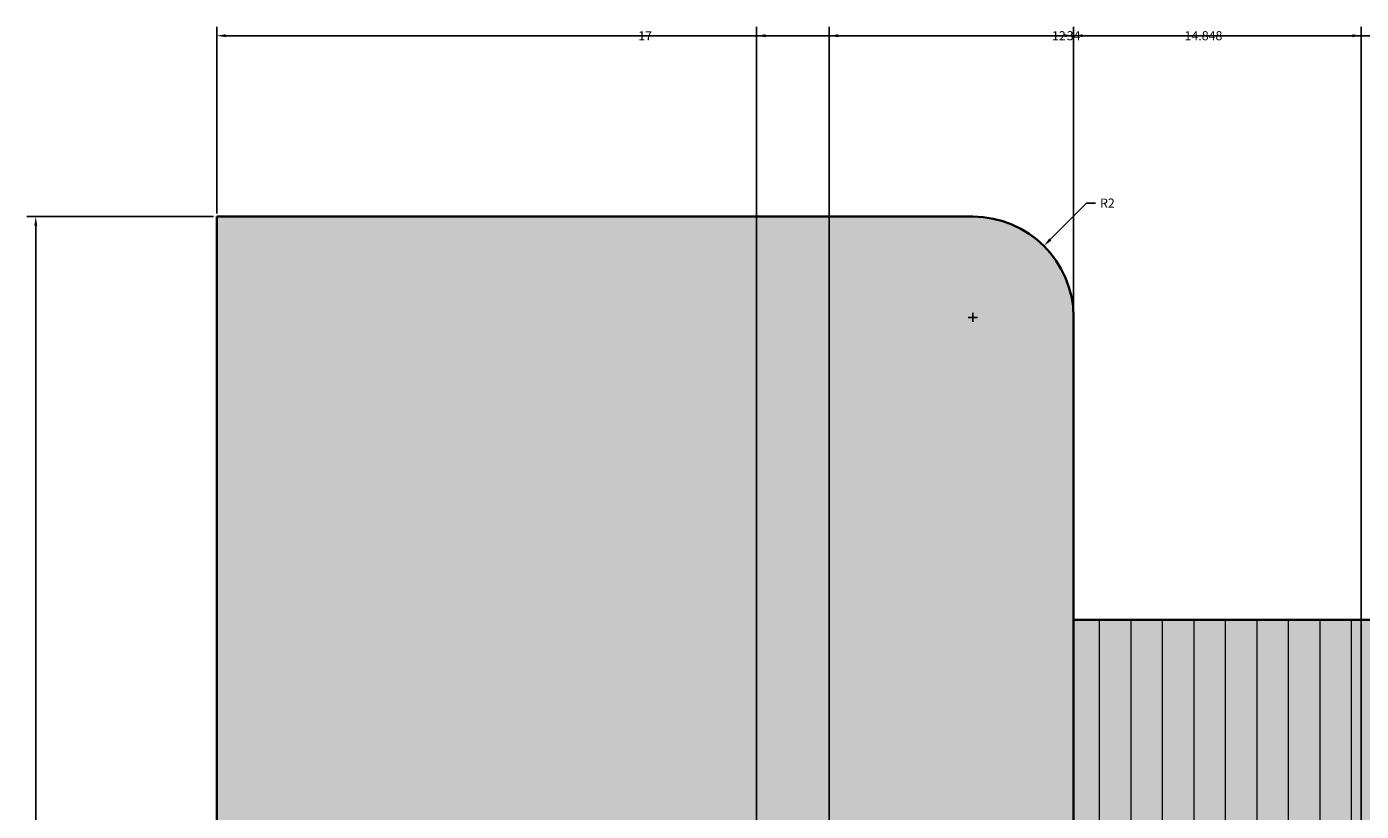
# Model space of a CAD drawing. Units: inches. Extents: x 18 to 59.8, y 2.7 to 81.2.
# Tile 8 of 9: x 18.1 to 44.6, y 65.6 to 81.2. Entities that reach past the tile are written whole.
import ezdxf

# ---------------------------------------------------------------- set-up
doc = ezdxf.new("R2010")
doc.units = ezdxf.units.IN
doc.header["$MEASUREMENT"] = 0
for name, color, linetype, lineweight in [('A-ANNO-DIMS', 2, 'Continuous', 18), ('A-ELEV', 7, 'Continuous', 35), ('A-ELEV-PATT', 8, 'Continuous', 13)]:
    doc.layers.add(name, color=color, linetype=linetype, lineweight=lineweight)
doc.styles.get("Standard").update_dxf_attribs({"font": 'arial.ttf'})
doc.dimstyles.get("Standard").update_dxf_attribs({"dimtxt": 0.18, "dimasz": 0.18, "dimexe": 0.18, "dimexo": 0.0625, "dimgap": 0.09, "dimtad": 0, "dimtih": 1, "dimtoh": 1, "dimdec": 1, "dimzin": 0, "dimdsep": 46, "dimlunit": 3, "dimtxsty": 'Standard', "dimcen": 0.09, "dimadec": 0, "dimazin": 0, "dimtfac": 1, "dimtdec": 1, "dimtofl": 0, "dimtmove": 0, "dimatfit": 3, "dimfxl": 1, "dimtolj": 1, "dimtzin": 0, "dimarcsym": 0})

# ---------------------------------------------------------------- blocks, each defined once
blk = doc.blocks.new('*D10')
at = {"layer": 'A-ANNO-DIMS', "color": 0, "lineweight": -2, "transparency": 16777216}
for p, q in [((21.86, 77.503), (21.86, 81.211)), ((22.04, 81.031), (38.641, 81.031)), ((55.68, 81.031), (39.078, 81.031)), ((55.86, 77.503), (55.86, 81.211))]:
    blk.add_line(p, q, dxfattribs=at)
at = {"layer": 'A-ANNO-DIMS', "color": 0, "transparency": 16777216}
for points in [[(22.04, 81.061), (22.04, 81.001), (21.86, 81.031)], [(55.68, 81.061), (55.68, 81.001), (55.86, 81.031)]]:
    blk.add_solid(points, dxfattribs=at)
at = {"layer": 'Defpoints', "color": 0, "transparency": 16777216}
for p in [(55.86, 81.031), (21.86, 77.441), (55.86, 77.441)]:
    blk.add_point(p, dxfattribs=at)
at = {"layer": 'A-ANNO-DIMS', "color": 0, "transparency": 16777216, "insert": (38.86, 81.031), "char_height": 0.18, "attachment_point": 5}
blk.add_mtext('\\A1;34', dxfattribs=at)
blk = doc.blocks.new('*D11')
at = {"layer": 'A-ANNO-DIMS', "color": 0, "lineweight": -2, "transparency": 16777216}
for p, q in [((21.86, 77.503), (21.86, 81.211)), ((22.04, 81.031), (30.15, 81.031)), ((38.68, 81.031), (30.57, 81.031)), ((38.86, 75.515), (38.86, 81.211))]:
    blk.add_line(p, q, dxfattribs=at)
at = {"layer": 'A-ANNO-DIMS', "color": 0, "transparency": 16777216}
for points in [[(22.04, 81.061), (22.04, 81.001), (21.86, 81.031)], [(38.68, 81.061), (38.68, 81.001), (38.86, 81.031)]]:
    blk.add_solid(points, dxfattribs=at)
at = {"layer": 'Defpoints', "color": 0, "transparency": 16777216}
for p in [(38.86, 81.031), (21.86, 77.441), (38.86, 75.452)]:
    blk.add_point(p, dxfattribs=at)
at = {"layer": 'A-ANNO-DIMS', "color": 0, "transparency": 16777216, "insert": (30.36, 81.031), "char_height": 0.18, "attachment_point": 5}
blk.add_mtext('\\A1;17', dxfattribs=at)
blk = doc.blocks.new('*D12')
at = {"layer": 'A-ANNO-DIMS', "color": 0, "lineweight": -2, "transparency": 16777216}
for p, q in [((38.86, 69.503), (38.86, 81.211)), ((39.04, 81.031), (45.765, 81.031)), ((53.26, 81.031), (46.535, 81.031)), ((53.44, 69.503), (53.44, 81.211))]:
    blk.add_line(p, q, dxfattribs=at)
at = {"layer": 'A-ANNO-DIMS', "color": 0, "transparency": 16777216}
for points in [[(39.04, 81.061), (39.04, 81.001), (38.86, 81.031)], [(53.26, 81.061), (53.26, 81.001), (53.44, 81.031)]]:
    blk.add_solid(points, dxfattribs=at)
at = {"layer": 'Defpoints', "color": 0, "transparency": 16777216}
for p in [(53.44, 81.031), (38.86, 69.441), (53.44, 69.441)]:
    blk.add_point(p, dxfattribs=at)
at = {"layer": 'A-ANNO-DIMS', "color": 0, "transparency": 16777216, "insert": (46.15, 81.031), "char_height": 0.18, "attachment_point": 5}
blk.add_mtext('\\A1;14.58', dxfattribs=at)
blk = doc.blocks.new('*D14')
at = {"layer": 'A-ANNO-DIMS', "color": 0, "lineweight": -2, "transparency": 16777216}
for p, q in [((21.797, 77.441), (18.09, 77.441)), ((18.27, 77.261), (18.27, 42.121)), ((18.27, 6.621), (18.27, 41.76)), ((21.797, 6.441), (18.09, 6.441))]:
    blk.add_line(p, q, dxfattribs=at)
at = {"layer": 'A-ANNO-DIMS', "color": 0, "transparency": 16777216}
for points in [[(18.24, 77.261), (18.3, 77.261), (18.27, 77.441)], [(18.24, 6.621), (18.3, 6.621), (18.27, 6.441)]]:
    blk.add_solid(points, dxfattribs=at)
at = {"layer": 'Defpoints', "color": 0, "transparency": 16777216}
for p in [(18.27, 77.441), (21.86, 77.441), (21.86, 6.441)]:
    blk.add_point(p, dxfattribs=at)
at = {"layer": 'A-ANNO-DIMS', "color": 0, "transparency": 16777216, "insert": (18.27, 41.941), "char_height": 0.18, "attachment_point": 5}
blk.add_mtext('\\A1;71', dxfattribs=at)
blk = doc.blocks.new('*D51')
at = {"layer": 'A-ANNO-DIMS', "color": 0, "lineweight": -2, "transparency": 16777216}
for p, q in [((34.012, 44.503), (34.012, 81.211)), ((34.192, 81.031), (40.98, 81.031)), ((48.68, 81.031), (41.891, 81.031)), ((48.86, 43.503), (48.86, 81.211))]:
    blk.add_line(p, q, dxfattribs=at)
at = {"layer": 'A-ANNO-DIMS', "color": 0, "transparency": 16777216}
for points in [[(34.192, 81.061), (34.192, 81.001), (34.012, 81.031)], [(48.68, 81.061), (48.68, 81.001), (48.86, 81.031)]]:
    blk.add_solid(points, dxfattribs=at)
at = {"layer": 'Defpoints', "color": 0, "transparency": 16777216}
for p in [(48.86, 81.031), (34.012, 44.441), (48.86, 43.441)]:
    blk.add_point(p, dxfattribs=at)
at = {"layer": 'A-ANNO-DIMS', "color": 0, "transparency": 16777216, "insert": (41.436, 81.031), "char_height": 0.18, "attachment_point": 5}
blk.add_mtext('\\A1;14.848', dxfattribs=at)
blk = doc.blocks.new('*D62')
at = {"layer": 'A-ANNO-DIMS', "color": 0, "lineweight": -2, "transparency": 16777216}
for p, q in [((32.567, 57.203), (32.567, 81.211)), ((32.747, 81.031), (38.358, 81.031)), ((44.387, 81.031), (38.777, 81.031)), ((44.567, 57.203), (44.567, 81.211))]:
    blk.add_line(p, q, dxfattribs=at)
at = {"layer": 'A-ANNO-DIMS', "color": 0, "transparency": 16777216}
for points in [[(32.747, 81.061), (32.747, 81.001), (32.567, 81.031)], [(44.387, 81.061), (44.387, 81.001), (44.567, 81.031)]]:
    blk.add_solid(points, dxfattribs=at)
at = {"layer": 'Defpoints', "color": 0, "transparency": 16777216}
for p in [(44.567, 81.031), (32.567, 57.141), (44.567, 57.141)]:
    blk.add_point(p, dxfattribs=at)
at = {"layer": 'A-ANNO-DIMS', "color": 0, "transparency": 16777216, "insert": (38.567, 81.031), "char_height": 0.18, "attachment_point": 5}
blk.add_mtext('\\A1;12', dxfattribs=at)
blk = doc.blocks.new('*D67')
at = {"layer": 'A-ANNO-DIMS', "color": 0, "lineweight": -2, "transparency": 16777216}
for p, q in [((39.116, 77.71), (38.397, 76.987)), ((39.296, 77.71), (39.116, 77.71)), ((36.86, 75.351), (36.86, 75.531)), ((36.77, 75.441), (36.95, 75.441))]:
    blk.add_line(p, q, dxfattribs=at)
at = {"layer": 'A-ANNO-DIMS', "color": 0, "transparency": 16777216}
blk.add_solid([(38.376, 77.008), (38.418, 76.966), (38.27, 76.859)], dxfattribs=at)
at = {"layer": 'Defpoints', "color": 0, "transparency": 16777216}
for p in [(38.27, 76.859), (36.86, 75.441)]:
    blk.add_point(p, dxfattribs=at)
at = {"layer": 'A-ANNO-DIMS', "color": 0, "transparency": 16777216, "insert": (39.53, 77.71), "char_height": 0.18, "attachment_point": 5}
blk.add_mtext('\\A1;R2', dxfattribs=at)

msp = doc.modelspace()

# ---------------------------------------------------------------- hatches: boundary and pattern name
at = {"layer": 'A-ELEV-PATT'}
h = msp.add_hatch(color=256, dxfattribs=at)
h.set_gradient(color1=(255, 255, 255), color2=(199, 200, 202))
h.paths.add_polyline_path([(38.86, 75.4521, 0.4125527), (36.86, 77.4407), (21.86, 77.4407), (21.86, 22.4407), (22.86, 22.4407), (48.86, 22.4407), (48.86, 30.9234, 0.4074473), (48.3302, 31.4407), (30.4061, 31.4407, -0.7603989), (34.0116, 44.4407), (47.86, 44.4407, -0.4142136), (48.86, 43.4407), (48.86, 48.4407, 0.4142136), (47.86, 49.4407), (32.2338, 49.4407, -0.2243142), (27.8411, 52.8427, -0.8480129), (38.86, 61.4407)])
h.paths.add_polyline_path([(55.86, 77.4407), (54.86, 77.4407), (54.86, 22.2407), (55.86, 22.2407)])
h.paths.add_polyline_path([(54.86, 51.5407), (53.4401, 51.5407), (53.4401, 29.6407), (54.86, 29.6407)])
h.paths.add_polyline_path([(54.86, 61.4407), (53.4401, 57.4407), (53.4401, 51.6407), (54.86, 51.6407)])
h.paths.add_polyline_path([(54.86, 29.4407), (54.471, 29.4407), (54.471, 22.2407), (54.86, 22.2407)])
h.paths.add_polyline_path([(55.5745, 22.2407), (54.86, 22.2407), (54.5745, 22.2407), (53.9347, 21.7925), (54.5877, 21.5495)])
h.paths.add_polyline_path([(54.5991, 21.5452), (53.9443, 21.789), (53.9443, 18.4407), (54.5991, 18.4407)])
h.paths.add_polyline_path([(53.9443, 21.789), (53.9347, 21.7925), (53.5816, 21.5452), (53.5816, 18.4407), (53.9443, 18.4407)])
h.paths.add_polyline_path([(53.3648, 20.6928), (52.8956, 21.0646), (52.8956, 18.4407), (53.3648, 18.4407)])
h.paths.add_polyline_path([(52.8956, 21.0646), (50.5775, 19.4407), (50.5775, 18.4407), (52.8956, 18.4407)])
h.paths.add_polyline_path([(53.5816, 21.5452), (52.8956, 21.0646), (53.3648, 20.6928), (53.5816, 20.8447)])
h.paths.add_polyline_path([(26.8109, 19.4407), (24.9672, 20.8407), (24.9672, 18.4407), (26.8109, 18.4407)])
h.paths.add_polyline_path([(24.9672, 20.8407), (24.4165, 20.8427), (24.4165, 18.4407), (24.9672, 18.4407)])
h.paths.add_polyline_path([(24.4165, 20.8427), (24.4165, 21.2589), (24.0588, 21.5305), (24.0301, 21.5183), (24.0301, 18.4407), (24.4165, 18.4407)])
h.paths.add_polyline_path([(24.0301, 21.5183), (23.4165, 21.2589), (23.4165, 18.4407), (24.0301, 18.4407)])
h.paths.add_polyline_path([(24.0301, 21.5183), (24.0588, 21.5305), (23.1234, 22.2407), (22.1234, 22.2407), (23.4165, 21.2589)])
h.paths.add_polyline_path([(24.4165, 21.2589), (24.4165, 20.8427), (24.9672, 20.8407)])
h.paths.add_polyline_path([(47.86, 18.4407), (29.86, 18.4407), (29.86, 6.4407), (30.86, 6.4407), (30.86, 17.4407), (38.86, 17.4407), (46.86, 17.4407), (46.86, 6.4407), (47.86, 6.4407)])
h.paths.add_polyline_path([(54.5756, 15.215), (54.5756, 6.4407), (55.86, 6.4407), (55.86, 18.4407), (47.86, 18.4407), (47.86, 6.4407), (49.1482, 6.4407), (49.1482, 15.215, -1)])
h = msp.add_hatch(color=256, dxfattribs=at)
h.dxf.hatch_style = 1
h.paths.add_polyline_path([(54.86, 69.4407), (38.86, 69.4407), (38.86, 61.4407), (54.86, 61.4407)])
h.paths.add_polyline_path([(54.86, 61.4407), (38.86, 61.4407), (36.86, 61.4407, 0.443414), (27.6986, 58.4407), (48.86, 58.4407), (48.86, 57.4407), (53.4401, 57.4407)])
h.paths.add_polyline_path([(37.4994, 59.9399), (37.4994, 59.8198, -2.4106499), (37.1187, 59.8198), (37.1187, 59.9399)], flags=16)
h.paths.add_polyline_path([(42.6125, 59.8012), (42.6125, 59.9213), (42.9933, 59.9213), (42.9933, 59.8012, -2.4106499)], flags=16)
h.paths.add_polyline_path([(49.5965, 59.971), (49.5965, 60.091), (49.9773, 60.091), (49.9773, 59.971, -2.4106499)], flags=16)
h.paths.add_polyline_path([(44.4671, 57.0407), (32.6671, 57.0407), (32.6671, 56.0407), (44.4671, 56.0407)])
h.paths.add_polyline_path([(47.86, 43.4407), (46.86, 43.4407), (34.0116, 43.4407, 0.2012983), (29.3481, 41.4407), (47.86, 41.4407, 1)])
h.paths.add_polyline_path([(36.5542, 42.5145), (36.5542, 42.6346), (36.9349, 42.6346), (36.9349, 42.5145, -2.4106499)], flags=16)
h.paths.add_polyline_path([(42.939, 42.5402), (42.939, 42.6603), (43.3198, 42.6603), (43.3198, 42.5402, -2.4106499)], flags=16)
h.paths.add_polyline_path([(54.471, 29.4407), (48.86, 29.4407), (48.86, 22.2407), (54.471, 22.2407)])
h.paths.add_polyline_path([(54.5745, 22.2407), (23.1234, 22.2407), (26.8109, 19.4407), (50.5775, 19.4407)])
h.paths.add_polyline_path([(54.5756, 15.215, 1), (49.1482, 15.215), (49.1482, 6.4407), (54.5756, 6.4407)])
h.paths.add_polyline_path([(49.8323, 12.602), (49.8323, 9.1225), (49.6657, 9.1225), (49.6657, 12.602)], flags=16)
h = msp.add_hatch(dxfattribs=at)
h.set_pattern_fill('ANSI31', color=256, scale=5, angle=45, style=0)
h.paths.add_polyline_path([(54.86, 69.4407), (38.86, 69.4407), (38.86, 61.4407), (54.86, 61.4407)])
h.paths.add_polyline_path([(54.86, 61.4407), (38.86, 61.4407), (36.86, 61.4407, 0.443414), (27.6986, 58.4407), (48.86, 58.4407), (48.86, 57.4407), (53.4401, 57.4407)])
h.paths.add_polyline_path([(37.1661, 59.8577), (37.1187, 59.8577), (37.1187, 59.9399), (37.4994, 59.9399), (37.4994, 59.8577), (37.452, 59.8577, -3.476462)], flags=16)
h.paths.add_polyline_path([(42.66, 59.8391), (42.6125, 59.8391), (42.6125, 59.9213), (42.9933, 59.9213), (42.9933, 59.8391), (42.9458, 59.8391, -3.476462)], flags=16)
h.paths.add_polyline_path([(49.644, 60.0088), (49.5965, 60.0088), (49.5965, 60.091), (49.9773, 60.091), (49.9773, 60.0088), (49.9298, 60.0088, -3.476462)], flags=16)
h.paths.add_polyline_path([(44.4671, 57.0407), (32.6671, 57.0407), (32.6671, 56.0407), (44.4671, 56.0407)])
h.paths.add_polyline_path([(47.86, 43.4407), (46.86, 43.4407), (34.0116, 43.4407, 0.2012983), (29.3481, 41.4407), (47.86, 41.4407, 1)])
h.paths.add_polyline_path([(36.6016, 42.5524), (36.5542, 42.5524), (36.5542, 42.6346), (36.9349, 42.6346), (36.9349, 42.5524), (36.8875, 42.5524, -3.476462)], flags=16)
h.paths.add_polyline_path([(42.9865, 42.578), (42.939, 42.578), (42.939, 42.6603), (43.3198, 42.6603), (43.3198, 42.578), (43.2723, 42.578, -3.476462)], flags=16)
h.paths.add_polyline_path([(54.471, 29.4407), (48.86, 29.4407), (48.86, 22.2407), (54.471, 22.2407)])
h.paths.add_polyline_path([(54.5745, 22.2407), (23.1234, 22.2407), (26.8109, 19.4407), (50.5775, 19.4407)])
h.paths.add_polyline_path([(54.5756, 15.215, 1), (49.1482, 15.215), (49.1482, 6.4407), (54.5756, 6.4407)])
h.paths.add_polyline_path([(49.8323, 9.1225), (49.6657, 9.1225), (49.6657, 12.602), (49.8323, 12.602)], flags=16)

# ---------------------------------------------------------------- linework, layer by layer
at = {"layer": 'A-ELEV'}
for p, q in [((21.86, 22.2407), (21.86, 77.4407)), ((36.86, 77.4407), (21.86, 77.4407)), ((36.86, 77.4407), (36.86, 77.4407)), ((38.86, 61.4407), (38.86, 75.4521)), ((54.86, 69.4407), (38.86, 69.4407))]:
    msp.add_line(p, q, dxfattribs=at)
msp.add_arc((36.86, 75.4407), 2, 0.32602, 90.00093, dxfattribs=at)

# ---------------------------------------------------------------- dimensions: what is measured, and where the dimension line sits
at = {"layer": 'A-ANNO-DIMS'}
for base, p1, p2, override, picture, middle in [((55.86, 81.0307), (21.86, 77.4407), (55.86, 77.4407), {"dimdec": 0, "dimlfac": 1, "dimrnd": 0, "dimzin": 0, "dimdsep": 46, "dimlunit": 2}, '*D10', (38.86, 81.0307)), ((38.86, 81.0307), (21.86, 77.4407), (38.86, 75.4521), {"dimdec": 0, "dimlfac": 1, "dimrnd": 0, "dimzin": 0, "dimdsep": 46, "dimlunit": 2}, '*D11', (30.36, 81.0307)), ((44.5671, 81.0307), (32.5671, 57.1407), (44.5671, 57.1407), {"dimdec": 0, "dimlfac": 1, "dimrnd": 0, "dimzin": 0, "dimdsep": 46, "dimlunit": 2}, '*D62', (38.5671, 81.0307)), ((48.86, 81.0307), (34.0116, 44.4407), (48.86, 43.4407), {"dimdec": 3, "dimlfac": 1, "dimrnd": 0, "dimzin": 0, "dimdsep": 46, "dimlunit": 2}, '*D51', (41.4358, 81.0307)), ((53.4401, 81.0307), (38.86, 69.4407), (53.4401, 69.4407), {"dimdec": 2, "dimlfac": 1, "dimrnd": 0, "dimzin": 0, "dimdsep": 46, "dimlunit": 2}, '*D12', (46.15, 81.0307))]:
    dim = msp.add_linear_dim(base=base, p1=p1, p2=p2, dimstyle='Standard', override=override, dxfattribs=at)
    dim.commit()
    dim.dimension.update_dxf_attribs({"geometry": picture, "text_midpoint": middle})
dim = msp.add_radius_dim(center=(36.86, 75.4407), mpoint=(38.2701, 76.8591), dimstyle='Standard', override={"dimdec": 0, "dimlfac": 1, "dimrnd": 0, "dimzin": 0, "dimdsep": 46, "dimlunit": 2}, dxfattribs=at)
dim.commit()
dim.dimension.update_dxf_attribs({"geometry": '*D67', "text_midpoint": (39.5303, 77.7101), "dimtype": 164})
dim = msp.add_linear_dim(base=(18.27, 77.4407), p1=(21.86, 6.4407), p2=(21.86, 77.4407), angle=90, dimstyle='Standard', override={"dimdec": 0, "dimlfac": 1, "dimrnd": 0, "dimzin": 0, "dimdsep": 46, "dimlunit": 2}, dxfattribs=at)
dim.commit()
dim.dimension.update_dxf_attribs({"geometry": '*D14', "text_midpoint": (18.27, 41.9407)})

doc.saveas('drawing.dxf')
